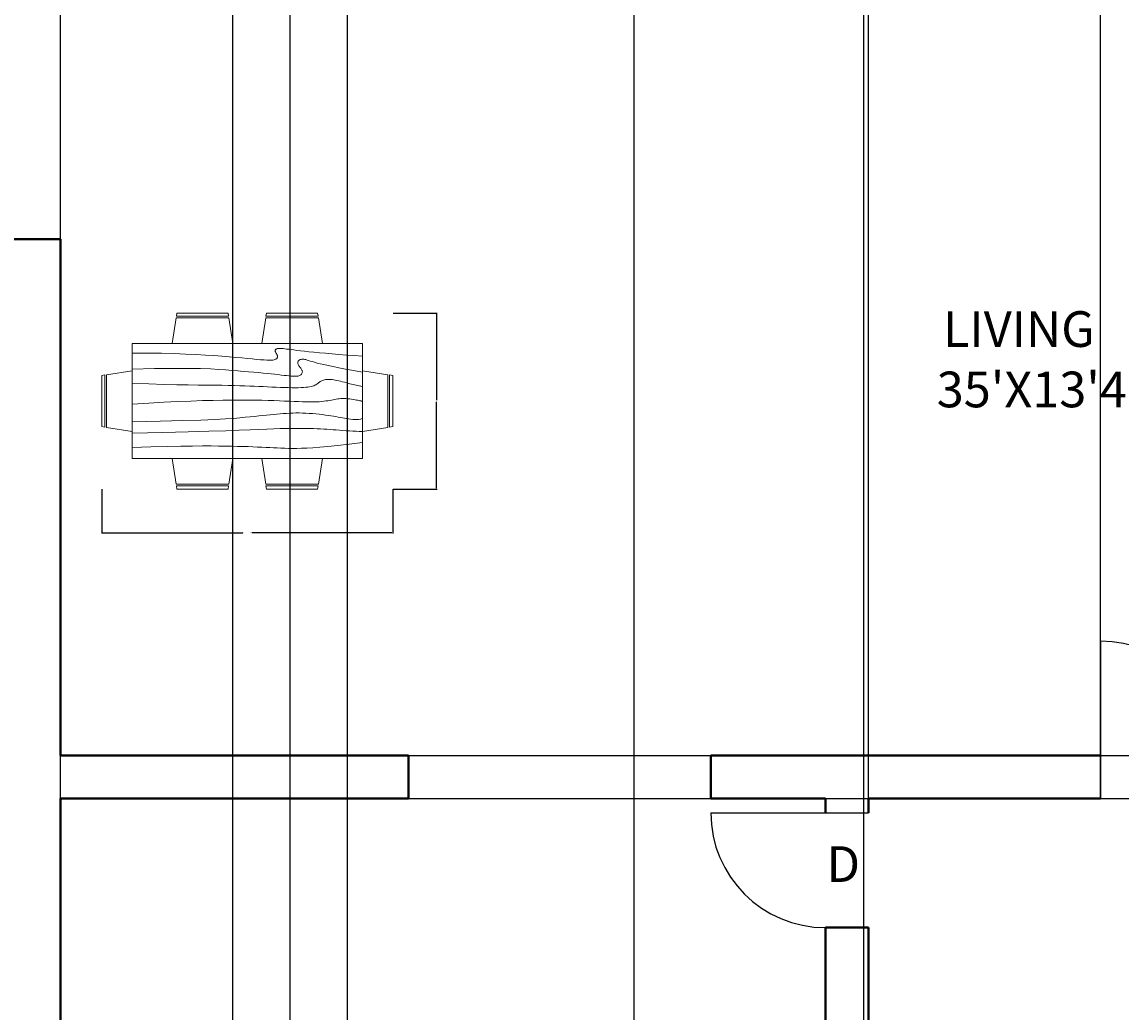
# Model space of a CAD drawing. Units: feet. Extents: x 2032 to 2763, y 1402 to 2145.
# Tile 4 of 6: x 2285 to 2515, y 1731 to 1938. Entities that reach past the tile are written whole.
import ezdxf

# ---------------------------------------------------------------- set-up
doc = ezdxf.new("R2010")
doc.units = ezdxf.units.FT
for name, color, linetype, lineweight in [('A-ANNO-DIMS', 2, 'Continuous', 18), ('A-ANNO-TEXT', 7, 'Continuous', 18), ('A-AREA-IDEN', 7, 'Continuous', 25), ('A-DOOR', 3, 'Continuous', 25), ('A-FURN', 8, 'Continuous', 18), ('A-WALL', 7, 'Continuous', 40)]:
    doc.layers.add(name, color=color, linetype=linetype, lineweight=lineweight)
doc.styles.get("Standard").update_dxf_attribs({"font": 'arial.ttf'})
doc.dimstyles.get("Standard").update_dxf_attribs({"dimtxt": 0.18, "dimasz": 0.18, "dimexe": 0.18, "dimexo": 0.0625, "dimgap": 0.09, "dimtad": 0, "dimtih": 1, "dimtoh": 1, "dimdec": 4, "dimzin": 0, "dimdsep": 46, "dimtxsty": 'Standard', "dimcen": 0.09, "dimadec": 0, "dimazin": 0, "dimtfac": 1, "dimtdec": 4, "dimtofl": 0, "dimtmove": 0, "dimatfit": 3, "dimfxl": 1, "dimtolj": 1, "dimtzin": 0, "dimarcsym": 0})

# ---------------------------------------------------------------- blocks, each defined once
blk = doc.blocks.new('Dining Set - 36 x 72 in.')
for p, q in [((-22.2343, 26.00059), (-23.4847, 17.99762)), ((-22.2304, 26), (-5.7608, 26)), ((-22, 27.5), (-22.1562, 26.50042)), ((-5.8416, 26.5), (-22.1534, 26.5)), ((-22, 27.5), (-6, 27.5)), ((-5.8437, 26.49966), (-6, 27.5)), ((-4.5152, 17.99762), (-5.7655, 25.99926)), ((5.7657, 26.00059), (4.5153, 17.99762)), ((5.7696, 26), (22.2392, 26)), ((6, 27.5), (5.8438, 26.50042)), ((22.1584, 26.5), (5.8466, 26.5)), ((6, 27.5), (22, 27.5)), ((22.1563, 26.49966), (22, 27.5)), ((23.4848, 17.99762), (22.2345, 25.99926)), ((36, 18), (-36, 18)), ((-36, 18), (-36, -18)), ((36, -18), (36, 18)), ((-45.5, 8), (-44.5004, 8.15617)), ((-45.5, 8), (-45.5, -8)), ((-44.5, -8.15843), (-44.5, 8.15338)), ((-44.0006, 8.23428), (-35.9976, 9.48474)), ((-44, 8.23041), (-44, -8.23915)), ((44.0006, 8.23428), (35.9976, 9.48474)), ((44, 8.23041), (44, -8.23915)), ((44.5, -8.15843), (44.5, 8.15338)), ((45.5, 8), (44.5005, 8.15617)), ((45.5, 8), (45.5, -8)), ((-44.4997, -8.15631), (-45.5, -8)), ((-35.9976, -9.48476), (-43.9993, -8.2345)), ((35.9976, -9.48476), (43.9993, -8.2345)), ((44.4997, -8.15631), (45.5, -8)), ((-36, -18), (36, -18)), ((-22.2343, -26.0006), (-23.4847, -17.99762)), ((-4.5152, -17.99762), (-5.7655, -25.99928)), ((5.7657, -26.0006), (4.5153, -17.99762)), ((23.4848, -17.99762), (22.2345, -25.99928)), ((-22.2304, -26), (-5.7608, -26)), ((-22, -27.5), (-22.1562, -26.50044)), ((-5.8416, -26.5), (-22.1534, -26.5)), ((-22, -27.5), (-6, -27.5)), ((-5.8437, -26.49967), (-6, -27.5)), ((5.7696, -26), (22.2392, -26)), ((6, -27.5), (5.8438, -26.50044)), ((22.1584, -26.5), (5.8466, -26.5)), ((6, -27.5), (22, -27.5)), ((22.1563, -26.49967), (22, -27.5))]:
    blk.add_line(p, q)
for points in [[(-36, 15), (-31.1772, 14.97754), (-26.8079, 14.91406), (-22.8538, 14.81543), (-19.276, 14.6875), (-16.0362, 14.53613), (-13.0957, 14.36718), (-10.4159, 14.18652), (-7.9583, 14), (-5.6904, 13.81315), (-3.6035, 13.63021), (-1.6954, 13.45508), (0.0365, 13.29166), (1.5945, 13.14388), (2.9811, 13.01562), (4.1988, 12.9108), (5.25, 12.83333), (6.1393, 12.78613), (6.8802, 12.76823), (7.4883, 12.77767), (7.9792, 12.8125), (8.3685, 12.87077), (8.6719, 12.95052), (8.9049, 13.0498), (9.0833, 13.16666), (9.2205, 13.29899), (9.3216, 13.44401), (9.3895, 13.59879), (9.4271, 13.76041), (9.4373, 13.92594), (9.4232, 14.09245), (9.3875, 14.257), (9.3333, 14.41666), (9.2638, 14.56917), (9.1836, 14.71484), (9.0975, 14.85465), (9.0104, 14.98958), (8.9272, 15.1206), (8.8529, 15.2487), (8.7922, 15.37483), (8.75, 15.5), (8.7305, 15.62467), (8.7344, 15.74739), (8.7617, 15.86621), (8.8125, 15.97916), (8.8867, 16.08431), (8.9844, 16.17968), (9.1055, 16.26334), (9.25, 16.33333), (9.4189, 16.38802), (9.6172, 16.42708), (9.8506, 16.45052), (10.125, 16.45833), (10.4463, 16.45052), (10.8203, 16.42708), (11.2529, 16.38802), (11.75, 16.33333), (12.3184, 16.26318), (12.9694, 16.17838), (13.7151, 16.07991), (14.5677, 15.96875), (15.5395, 15.84586), (16.6426, 15.71224), (17.8893, 15.56884), (19.2917, 15.41666), (20.859, 15.25667), (22.5879, 15.08984), (24.4721, 14.91715), (26.5052, 14.73958), (28.6809, 14.5581), (30.9929, 14.3737), (33.4347, 14.18733), (36, 14)], [(-36, 10), (-28.9766, 10.14274), (-23.1725, 10.20442), (-18.4241, 10.19775), (-14.5677, 10.13541), (-11.4399, 10.03011), (-8.877, 9.89453), (-6.7154, 9.74137), (-4.7917, 9.58333), (-2.9698, 9.43082), (-1.2246, 9.28515), (0.4415, 9.14534), (2.026, 9.01041), (3.5266, 8.87939), (4.9408, 8.7513), (6.266, 8.62516), (7.5, 8.5), (8.6411, 8.37549), (9.6914, 8.2539), (10.6538, 8.13818), (11.5312, 8.03125), (12.3267, 7.93603), (13.043, 7.85547), (13.6831, 7.79248), (14.25, 7.75), (14.7471, 7.7303), (15.1797, 7.73307), (15.5537, 7.75732), (15.875, 7.80208), (16.1494, 7.86637), (16.3828, 7.94922), (16.5811, 8.04964), (16.75, 8.16666), (16.8944, 8.29915), (17.0143, 8.44531), (17.1089, 8.60319), (17.1771, 8.77083), (17.218, 8.94629), (17.2305, 9.1276), (17.2137, 9.31282), (17.1667, 9.5), (17.0895, 9.6875), (16.987, 9.875), (16.8649, 10.0625), (16.7292, 10.25), (16.5856, 10.4375), (16.4401, 10.625), (16.2985, 10.8125), (16.1667, 11), (16.05, 11.18733), (15.9518, 11.3737), (15.8752, 11.5581), (15.8229, 11.73958), (15.798, 11.91715), (15.8034, 12.08984), (15.842, 12.25667), (15.9167, 12.41666), (16.0295, 12.56836), (16.1784, 12.70833), (16.3605, 12.83268), (16.5729, 12.9375), (16.8127, 13.01888), (17.0768, 13.07291), (17.3625, 13.0957), (17.6667, 13.08333), (17.9894, 13.03312), (18.3418, 12.94726), (18.7382, 12.82918), (19.1927, 12.68229), (19.7195, 12.51001), (20.3327, 12.31575), (21.0465, 12.10294), (21.875, 11.875), (22.8357, 11.63354), (23.959, 11.37304), (25.2786, 11.08618), (26.8282, 10.76562), (28.6414, 10.40405), (30.752, 9.99414), (33.1936, 9.52856), (36, 9)], [(-36, 5.5), (-30.7157, 5.3348), (-26.069, 5.20963), (-21.9946, 5.11767), (-18.4271, 5.05208), (-15.3009, 5.00602), (-12.5508, 4.97265), (-10.1112, 4.94515), (-7.9167, 4.91666), (-5.909, 4.88167), (-4.0586, 4.83984), (-2.3429, 4.79215), (-0.7396, 4.73958), (0.7739, 4.6831), (2.22, 4.6237), (3.6213, 4.56233), (5, 4.5), (6.373, 4.43782), (7.7344, 4.3776), (9.0723, 4.32129), (10.375, 4.27083), (11.6309, 4.22819), (12.8281, 4.19531), (13.9551, 4.17415), (15, 4.16666), (15.954, 4.17448), (16.819, 4.19791), (17.6001, 4.23698), (18.3021, 4.29166), (18.9299, 4.36198), (19.4883, 4.44791), (19.9823, 4.54948), (20.4167, 4.66666), (20.7969, 4.79899), (21.1302, 4.94401), (21.4245, 5.09879), (21.6875, 5.26041), (21.9271, 5.42594), (22.1511, 5.59245), (22.3672, 5.757), (22.5834, 5.91666), (22.8065, 6.06868), (23.0404, 6.21093), (23.2879, 6.34147), (23.5521, 6.45833), (23.8358, 6.55957), (24.142, 6.64323), (24.4735, 6.70735), (24.8334, 6.75), (25.2235, 6.76969), (25.642, 6.76692), (26.0858, 6.74267), (26.5521, 6.69791), (27.0379, 6.63362), (27.5404, 6.55078), (28.0565, 6.45036), (28.5834, 6.33333), (29.1242, 6.19987), (29.7071, 6.04687), (30.3661, 5.87044), (31.1354, 5.66666), (32.0493, 5.43164), (33.142, 5.16146), (34.4475, 4.85221), (36, 4.5)], [(-36, -1), (-30.7915, -0.6591), (-26.0195, -0.38216), (-21.6519, -0.16284), (-17.6563, 0.00521), (-14.0005, 0.12833), (-10.6523, 0.21289), (-7.5796, 0.26522), (-4.75, 0.29166), (-2.134, 0.29793), (0.2878, 0.28711), (2.5317, 0.26163), (4.6146, 0.22396), (6.5529, 0.17651), (8.3633, 0.12174), (10.0623, 0.06209), (11.6667, 0), (13.1899, -0.06201), (14.6341, -0.1211), (15.9982, -0.17432), (17.2813, -0.21875), (18.4823, -0.25147), (19.6003, -0.26953), (20.6343, -0.27002), (21.5834, -0.25), (22.4481, -0.20768), (23.2357, -0.14584), (23.9549, -0.06836), (24.6146, 0.02083), (25.2235, 0.11784), (25.7904, 0.21875), (26.3241, 0.31966), (26.8334, 0.41666), (27.3265, 0.50618), (27.8099, 0.58593), (28.2894, 0.65397), (28.7709, 0.70833), (29.2601, 0.74707), (29.763, 0.76823), (30.2855, 0.76985), (30.8334, 0.75), (31.4088, 0.70784), (31.9994, 0.64713), (32.589, 0.57275), (33.1615, 0.48958), (33.7008, 0.4025), (34.1908, 0.3164), (34.6153, 0.23616), (34.9584, 0.16666), (35.2099, 0.11165), (35.3848, 0.07031), (35.504, 0.04069), (35.5886, 0.02083), (35.6594, 0.00879), (35.7377, 0.0026), (35.8442, 0.00032), (36, 0)], [(-36, -6.5), (-27.1843, -6.31267), (-20.084, -6.1263), (-14.469, -5.9419), (-10.1094, -5.76042), (-6.7752, -5.58285), (-4.2363, -5.41016), (-2.2629, -5.24333), (-0.625, -5.08334), (0.8708, -4.93099), (2.2715, -4.78646), (3.5872, -4.64974), (4.8281, -4.52084), (6.0046, -4.39974), (7.127, -4.28646), (8.2053, -4.18099), (9.25, -4.08334), (10.2705, -3.99382), (11.2734, -3.91407), (12.2647, -3.84603), (13.25, -3.79167), (14.2354, -3.75293), (15.2266, -3.73177), (16.2295, -3.73015), (17.25, -3.75), (18.2912, -3.79248), (19.3451, -3.85547), (20.4009, -3.93604), (21.4479, -4.03125), (22.4754, -4.13819), (23.4727, -4.25391), (24.4289, -4.37549), (25.3334, -4.5), (26.1785, -4.62492), (26.9694, -4.74935), (27.7145, -4.87281), (28.4219, -4.99479), (29.1, -5.11483), (29.7572, -5.23242), (30.4016, -5.34709), (31.0417, -5.45834), (31.6837, -5.56437), (32.3262, -5.65821), (32.9658, -5.73153), (33.599, -5.77604), (34.2224, -5.78345), (34.8327, -5.74545), (35.4264, -5.65373), (36, -5.5)], [(-36, -10), (-26.4022, -9.81299), (-18.4675, -9.62891), (-11.9839, -9.45069), (-6.7396, -9.28125), (-2.5226, -9.12354), (0.8789, -8.98047), (3.6769, -8.85498), (6.0833, -8.75), (8.2767, -8.66765), (10.3021, -8.60677), (12.1712, -8.56543), (13.8958, -8.54167), (15.4876, -8.53353), (16.9583, -8.53907), (18.3197, -8.55632), (19.5834, -8.58334), (20.7616, -8.61841), (21.8685, -8.66081), (22.9188, -8.71004), (23.9271, -8.76563), (24.9081, -8.82707), (25.8763, -8.89388), (26.8465, -8.96558), (27.8334, -9.04167), (28.8474, -9.12118), (29.8828, -9.20117), (30.93, -9.27824), (31.9792, -9.34896), (33.0205, -9.40991), (34.0443, -9.45768), (35.0407, -9.48885), (36, -9.5)], [(-36, -14.5), (-30.0881, -14.33513), (-25.0332, -14.21224), (-20.7312, -14.12647), (-17.0781, -14.07292), (-13.97, -14.04671), (-11.3027, -14.04297), (-8.9724, -14.05681), (-6.875, -14.08334), (-4.9224, -14.11833), (-3.0905, -14.16016), (-1.3709, -14.20785), (0.2448, -14.26042), (1.7647, -14.3169), (3.1973, -14.3763), (4.5507, -14.43767), (5.8333, -14.5), (7.0554, -14.5621), (8.235, -14.62175), (9.3922, -14.67652), (10.5469, -14.72396), (11.7192, -14.76164), (12.929, -14.78711), (14.1965, -14.79794), (15.5417, -14.79167), (16.9933, -14.76424), (18.6152, -14.70508), (20.4804, -14.60197), (22.6615, -14.44271), (25.2312, -14.21509), (28.2624, -13.9069), (31.8277, -13.50594), (36, -13)]]:
    blk.add_lwpolyline(points)
blk = doc.blocks.new('DOOR-SWING-24')
blk.add_line((33, 0), (0, 0))
blk.add_arc((9, 0), 24, 0, 90)
blk = doc.blocks.new('*D31')
at = {"layer": 'A-ANNO-DIMS', "color": 0, "lineweight": -2, "transparency": 16777216}
for p, q in [((2301.9, 1840.29), (2301.9, 1831.04)), ((2362.79, 1840.29), (2362.79, 1831.04)), ((2302.08, 1831.22), (2331.39, 1831.22)), ((2362.61, 1831.22), (2333.3, 1831.22))]:
    blk.add_line(p, q, dxfattribs=at)
at = {"layer": 'A-ANNO-DIMS', "color": 0, "transparency": 16777216}
for points in [[(2302.08, 1831.25), (2302.08, 1831.19), (2301.9, 1831.22)], [(2362.61, 1831.25), (2362.61, 1831.19), (2362.79, 1831.22)]]:
    blk.add_solid(points, dxfattribs=at)
at = {"layer": 'Defpoints', "color": 0, "transparency": 16777216}
for p in [(2301.9, 1840.35), (2362.79, 1840.35), (2362.79, 1831.22)]:
    blk.add_point(p, dxfattribs=at)
at = {"layer": 'A-ANNO-DIMS', "color": 0, "transparency": 16777216, "insert": (2332.34, 1831.22), "char_height": 0.18, "attachment_point": 5}
blk.add_mtext('\\A1;DINING SET 61', dxfattribs=at)
blk = doc.blocks.new('*D32')
at = {"layer": 'A-ANNO-DIMS', "color": 0, "lineweight": -2, "transparency": 16777216}
for p, q in [((2362.85, 1877.15), (2372.1, 1877.15)), ((2371.92, 1876.97), (2371.92, 1858.93)), ((2371.92, 1840.53), (2371.92, 1858.57)), ((2362.85, 1840.35), (2372.1, 1840.35))]:
    blk.add_line(p, q, dxfattribs=at)
at = {"layer": 'A-ANNO-DIMS', "color": 0, "transparency": 16777216}
for points in [[(2371.89, 1876.97), (2371.95, 1876.97), (2371.92, 1877.15)], [(2371.89, 1840.53), (2371.95, 1840.53), (2371.92, 1840.35)]]:
    blk.add_solid(points, dxfattribs=at)
at = {"layer": 'Defpoints', "color": 0, "transparency": 16777216}
for p in [(2362.79, 1877.15), (2371.92, 1877.15), (2362.79, 1840.35)]:
    blk.add_point(p, dxfattribs=at)
at = {"layer": 'A-ANNO-DIMS', "color": 0, "transparency": 16777216, "insert": (2371.92, 1858.75), "char_height": 0.18, "attachment_point": 5}
blk.add_mtext('\\A1;37', dxfattribs=at)
blk = doc.blocks.new('*D67')
at = {"layer": 'A-ANNO-DIMS', "color": 0, "lineweight": -2, "transparency": 16777216}
for p, q in [((2329.31, 1594.68), (2329.31, 2145.29)), ((2329.49, 2145.11), (2395.03, 2145.11)), ((2461.13, 2145.11), (2395.59, 2145.11)), ((2461.31, 1594.68), (2461.31, 2145.29))]:
    blk.add_line(p, q, dxfattribs=at)
at = {"layer": 'A-ANNO-DIMS', "color": 0, "transparency": 16777216}
for points in [[(2329.49, 2145.14), (2329.49, 2145.08), (2329.31, 2145.11)], [(2461.13, 2145.14), (2461.13, 2145.08), (2461.31, 2145.11)]]:
    blk.add_solid(points, dxfattribs=at)
at = {"layer": 'Defpoints', "color": 0, "transparency": 16777216}
for p in [(2461.31, 2145.11), (2329.31, 1594.61), (2461.31, 1594.61)]:
    blk.add_point(p, dxfattribs=at)
at = {"layer": 'A-ANNO-DIMS', "color": 0, "transparency": 16777216, "insert": (2395.31, 2145.11), "char_height": 0.18, "attachment_point": 5}
blk.add_mtext('\\A1;132', dxfattribs=at)
blk = doc.blocks.new('*D69')
at = {"layer": 'A-ANNO-DIMS', "color": 0, "lineweight": -2, "transparency": 16777216}
for p, q in [((2341.31, 1505.68), (2341.31, 2145.29)), ((2341.49, 2145.11), (2347.1, 2145.11)), ((2353.13, 2145.11), (2347.52, 2145.11)), ((2353.31, 1505.68), (2353.31, 2145.29))]:
    blk.add_line(p, q, dxfattribs=at)
at = {"layer": 'A-ANNO-DIMS', "color": 0, "transparency": 16777216}
for points in [[(2341.49, 2145.14), (2341.49, 2145.08), (2341.31, 2145.11)], [(2353.13, 2145.14), (2353.13, 2145.08), (2353.31, 2145.11)]]:
    blk.add_solid(points, dxfattribs=at)
at = {"layer": 'Defpoints', "color": 0, "transparency": 16777216}
for p in [(2353.31, 2145.11), (2341.31, 1505.61), (2353.31, 1505.61)]:
    blk.add_point(p, dxfattribs=at)
at = {"layer": 'A-ANNO-DIMS', "color": 0, "transparency": 16777216, "insert": (2347.31, 2145.11), "char_height": 0.18, "attachment_point": 5}
blk.add_mtext('\\A1;12', dxfattribs=at)
blk = doc.blocks.new('*D72')
at = {"layer": 'A-ANNO-DIMS', "color": 0, "lineweight": -2, "transparency": 16777216}
for p, q in [((2293.31, 1505.68), (2293.31, 2145.29)), ((2293.49, 2145.11), (2311.09, 2145.11)), ((2329.13, 2145.11), (2311.53, 2145.11)), ((2329.31, 1501.18), (2329.31, 2145.29))]:
    blk.add_line(p, q, dxfattribs=at)
at = {"layer": 'A-ANNO-DIMS', "color": 0, "transparency": 16777216}
for points in [[(2293.49, 2145.14), (2293.49, 2145.08), (2293.31, 2145.11)], [(2329.13, 2145.14), (2329.13, 2145.08), (2329.31, 2145.11)]]:
    blk.add_solid(points, dxfattribs=at)
at = {"layer": 'Defpoints', "color": 0, "transparency": 16777216}
for p in [(2329.31, 2145.11), (2293.31, 1505.61), (2329.31, 1501.11)]:
    blk.add_point(p, dxfattribs=at)
at = {"layer": 'A-ANNO-DIMS', "color": 0, "transparency": 16777216, "insert": (2311.31, 2145.11), "char_height": 0.18, "attachment_point": 5}
blk.add_mtext('\\A1;36', dxfattribs=at)
blk = doc.blocks.new('*D73')
at = {"layer": 'A-ANNO-DIMS', "color": 0, "lineweight": -2, "transparency": 16777216}
for p, q in [((2462.31, 1775.68), (2462.31, 2145.29)), ((2462.49, 2145.11), (2486.24, 2145.11)), ((2510.63, 2145.11), (2486.89, 2145.11)), ((2510.81, 1775.68), (2510.81, 2145.29))]:
    blk.add_line(p, q, dxfattribs=at)
at = {"layer": 'A-ANNO-DIMS', "color": 0, "transparency": 16777216}
for points in [[(2462.49, 2145.14), (2462.49, 2145.08), (2462.31, 2145.11)], [(2510.63, 2145.14), (2510.63, 2145.08), (2510.81, 2145.11)]]:
    blk.add_solid(points, dxfattribs=at)
at = {"layer": 'Defpoints', "color": 0, "transparency": 16777216}
for p in [(2510.81, 2145.11), (2462.31, 1775.61), (2510.81, 1775.61)]:
    blk.add_point(p, dxfattribs=at)
at = {"layer": 'A-ANNO-DIMS', "color": 0, "transparency": 16777216, "insert": (2486.56, 2145.11), "char_height": 0.18, "attachment_point": 5}
blk.add_mtext('\\A1;48.5', dxfattribs=at)
blk = doc.blocks.new('*D74')
at = {"layer": 'A-ANNO-DIMS', "color": 0, "lineweight": -2, "transparency": 16777216}
for p, q in [((2510.81, 1775.68), (2510.81, 2145.29)), ((2510.99, 2145.11), (2534.59, 2145.11)), ((2558.63, 2145.11), (2535.04, 2145.11)), ((2558.81, 1775.68), (2558.81, 2145.29))]:
    blk.add_line(p, q, dxfattribs=at)
at = {"layer": 'A-ANNO-DIMS', "color": 0, "transparency": 16777216}
for points in [[(2510.99, 2145.14), (2510.99, 2145.08), (2510.81, 2145.11)], [(2558.63, 2145.14), (2558.63, 2145.08), (2558.81, 2145.11)]]:
    blk.add_solid(points, dxfattribs=at)
at = {"layer": 'Defpoints', "color": 0, "transparency": 16777216}
for p in [(2558.81, 2145.11), (2510.81, 1775.61), (2558.81, 1775.61)]:
    blk.add_point(p, dxfattribs=at)
at = {"layer": 'A-ANNO-DIMS', "color": 0, "transparency": 16777216, "insert": (2534.81, 2145.11), "char_height": 0.18, "attachment_point": 5}
blk.add_mtext('\\A1;48', dxfattribs=at)
blk = doc.blocks.new('*D79')
at = {"layer": 'A-ANNO-DIMS', "color": 0, "lineweight": -2, "transparency": 16777216}
for p, q in [((2353.31, 1603.68), (2353.31, 2145.29)), ((2353.49, 2145.11), (2383.09, 2145.11)), ((2413.13, 2145.11), (2383.53, 2145.11)), ((2413.31, 1603.68), (2413.31, 2145.29))]:
    blk.add_line(p, q, dxfattribs=at)
at = {"layer": 'A-ANNO-DIMS', "color": 0, "transparency": 16777216}
for points in [[(2353.49, 2145.14), (2353.49, 2145.08), (2353.31, 2145.11)], [(2413.13, 2145.14), (2413.13, 2145.08), (2413.31, 2145.11)]]:
    blk.add_solid(points, dxfattribs=at)
at = {"layer": 'Defpoints', "color": 0, "transparency": 16777216}
for p in [(2413.31, 2145.11), (2353.31, 1603.61), (2413.31, 1603.61)]:
    blk.add_point(p, dxfattribs=at)
at = {"layer": 'A-ANNO-DIMS', "color": 0, "transparency": 16777216, "insert": (2383.31, 2145.11), "char_height": 0.18, "attachment_point": 5}
blk.add_mtext('\\A1;60', dxfattribs=at)
blk = doc.blocks.new('*D81')
at = {"layer": 'A-ANNO-DIMS', "color": 0, "lineweight": -2, "transparency": 16777216}
for p, q in [((2293.31, 1603.68), (2293.31, 2145.29)), ((2293.49, 2145.11), (2323.09, 2145.11)), ((2353.13, 2145.11), (2323.53, 2145.11)), ((2353.31, 1603.68), (2353.31, 2145.29))]:
    blk.add_line(p, q, dxfattribs=at)
at = {"layer": 'A-ANNO-DIMS', "color": 0, "transparency": 16777216}
for points in [[(2293.49, 2145.14), (2293.49, 2145.08), (2293.31, 2145.11)], [(2353.13, 2145.14), (2353.13, 2145.08), (2353.31, 2145.11)]]:
    blk.add_solid(points, dxfattribs=at)
at = {"layer": 'Defpoints', "color": 0, "transparency": 16777216}
for p in [(2353.31, 2145.11), (2293.31, 1603.61), (2353.31, 1603.61)]:
    blk.add_point(p, dxfattribs=at)
at = {"layer": 'A-ANNO-DIMS', "color": 0, "transparency": 16777216, "insert": (2323.31, 2145.11), "char_height": 0.18, "attachment_point": 5}
blk.add_mtext('\\A1;60', dxfattribs=at)
blk = doc.blocks.new('*D82')
at = {"layer": 'A-ANNO-DIMS', "color": 0, "lineweight": -2, "transparency": 16777216}
for p, q in [((2293.38, 1784.61), (2762.99, 1784.61)), ((2762.81, 1784.43), (2762.81, 1780.29)), ((2762.81, 1775.79), (2762.81, 1779.93)), ((2293.38, 1775.61), (2762.99, 1775.61))]:
    blk.add_line(p, q, dxfattribs=at)
at = {"layer": 'A-ANNO-DIMS', "color": 0, "transparency": 16777216}
for points in [[(2762.78, 1784.43), (2762.84, 1784.43), (2762.81, 1784.61)], [(2762.78, 1775.79), (2762.84, 1775.79), (2762.81, 1775.61)]]:
    blk.add_solid(points, dxfattribs=at)
at = {"layer": 'Defpoints', "color": 0, "transparency": 16777216}
for p in [(2293.31, 1784.61), (2762.81, 1784.61), (2293.31, 1775.61)]:
    blk.add_point(p, dxfattribs=at)
at = {"layer": 'A-ANNO-DIMS', "color": 0, "transparency": 16777216, "insert": (2762.81, 1780.11), "char_height": 0.18, "attachment_point": 5}
blk.add_mtext('\\A1;9', dxfattribs=at)

msp = doc.modelspace()

# ---------------------------------------------------------------- linework, layer by layer
at = {"layer": 'A-WALL'}
for p, q in [((2293.3136, 1892.6131), (2282.3136, 1892.6131)), ((2293.3136, 1784.6131), (2293.3136, 1892.6131)), ((2366.0636, 1784.6131), (2293.3136, 1784.6131)), ((2366.0636, 1784.6131), (2366.0636, 1775.6131)), ((2510.8136, 1784.6131), (2429.3136, 1784.6131)), ((2429.3136, 1775.6131), (2429.3136, 1784.6131)), ((2293.3136, 1775.6131), (2293.3136, 1654.6686)), ((2366.0636, 1775.6131), (2293.3136, 1775.6131)), ((2453.3136, 1775.6131), (2429.3136, 1775.6131)), ((2453.3136, 1772.6131), (2453.3136, 1775.6131)), ((2510.8136, 1775.6131), (2462.3136, 1775.6131)), ((2462.3136, 1772.6131), (2462.3136, 1775.6131)), ((2453.3136, 1603.6131), (2453.3136, 1748.6131)), ((2462.3136, 1748.6131), (2453.3136, 1748.6131)), ((2462.3136, 1594.6131), (2462.3136, 1748.6131))]:
    msp.add_line(p, q, dxfattribs=at)

# ---------------------------------------------------------------- block references
at = {"layer": 'A-DOOR', "extrusion": (0, 0, -1), "zscale": -1, "rotation": 90.0000000000006}
msp.add_blockref('DOOR-SWING-24', (-2510.8136, 1775.6134), dxfattribs=at)
at = {"layer": 'A-DOOR', "rotation": 180}
msp.add_blockref('DOOR-SWING-24', (2462.3133, 1772.6131), dxfattribs=at)
at = {"layer": 'A-FURN', "xscale": 0.6691115677897082, "yscale": 0.6691115677897082, "zscale": 0.6691115677897082}
msp.add_blockref('Dining Set - 36 x 72 in.', (2332.3438, 1858.7495), dxfattribs=at)

# ---------------------------------------------------------------- texts
at = {"layer": 'A-ANNO-TEXT'}
msp.add_text('D', height=7.4682, dxfattribs=at).set_placement((2453.5166, 1758.1631))
at = {"layer": 'A-AREA-IDEN'}
for s, p in [('LIVING', (2477.8676, 1870.0688)), ('35\'X13\'4"', (2476.56, 1857.4415))]:
    msp.add_text(s, height=7.46821, dxfattribs=at).set_placement(p)

# ---------------------------------------------------------------- dimensions: what is measured, and where the dimension line sits
at = {"layer": 'A-ANNO-DIMS'}
for base, p1, p2, override, picture, middle in [((2329.3136, 2145.1131), (2293.3136, 1505.6131), (2329.3136, 1501.1131), {"dimdec": 0, "dimlfac": 1, "dimrnd": 0, "dimzin": 0, "dimdsep": 46, "dimlunit": 2}, '*D72', (2311.3136, 2145.1131)), ((2353.3136, 2145.1131), (2293.3136, 1603.6131), (2353.3136, 1603.6131), {"dimdec": 0, "dimlfac": 1, "dimrnd": 0, "dimzin": 0, "dimdsep": 46, "dimlunit": 2}, '*D81', (2323.3136, 2145.1131)), ((2461.3136, 2145.1131), (2329.3136, 1594.6131), (2461.3136, 1594.6131), {"dimdec": 0, "dimlfac": 1, "dimrnd": 0, "dimzin": 0, "dimdsep": 46, "dimlunit": 2}, '*D67', (2395.3136, 2145.1131)), ((2353.3136, 2145.1131), (2341.3136, 1505.6131), (2353.3136, 1505.6131), {"dimdec": 0, "dimlfac": 1, "dimrnd": 0, "dimzin": 0, "dimdsep": 46, "dimlunit": 2}, '*D69', (2347.3136, 2145.1131)), ((2413.3136, 2145.1131), (2353.3136, 1603.6131), (2413.3136, 1603.6131), {"dimdec": 0, "dimlfac": 1, "dimrnd": 0, "dimzin": 0, "dimdsep": 46, "dimlunit": 2}, '*D79', (2383.3136, 2145.1131)), ((2510.8136, 2145.1131), (2462.3136, 1775.6131), (2510.8136, 1775.6131), {"dimdec": 1, "dimlfac": 1, "dimrnd": 0, "dimzin": 0, "dimdsep": 46, "dimlunit": 2}, '*D73', (2486.5636, 2145.1131)), ((2558.8136, 2145.1131), (2510.8136, 1775.6131), (2558.8136, 1775.6131), {"dimdec": 0, "dimlfac": 1, "dimrnd": 0, "dimzin": 0, "dimdsep": 46, "dimlunit": 2}, '*D74', (2534.8136, 2145.1131))]:
    dim = msp.add_linear_dim(base=base, p1=p1, p2=p2, dimstyle='Standard', override=override, dxfattribs=at)
    dim.commit()
    dim.dimension.update_dxf_attribs({"geometry": picture, "text_midpoint": middle})
for base, p1, p2, picture, middle in [((2371.9218, 1877.1501), (2362.7884, 1840.3489), (2362.7884, 1877.1501), '*D32', (2371.9218, 1858.7495)), ((2762.8136, 1784.6131), (2293.3136, 1775.6131), (2293.3136, 1784.6131), '*D82', (2762.8136, 1780.1131))]:
    dim = msp.add_linear_dim(base=base, p1=p1, p2=p2, angle=90, dimstyle='Standard', override={"dimdec": 0, "dimlfac": 1, "dimrnd": 0, "dimzin": 0, "dimdsep": 46, "dimlunit": 2}, dxfattribs=at)
    dim.commit()
    dim.dimension.update_dxf_attribs({"geometry": picture, "text_midpoint": middle})
dim = msp.add_linear_dim(base=(2362.7884, 1831.2156), p1=(2301.8993, 1840.3489), p2=(2362.7884, 1840.3489), text='DINING SET <>', dimstyle='Standard', override={"dimdec": 0, "dimlfac": 1, "dimrnd": 0, "dimzin": 0, "dimdsep": 46, "dimlunit": 2}, dxfattribs=at)
dim.commit()
dim.dimension.update_dxf_attribs({"geometry": '*D31', "text_midpoint": (2332.3438, 1831.2156)})

doc.saveas('drawing.dxf')
